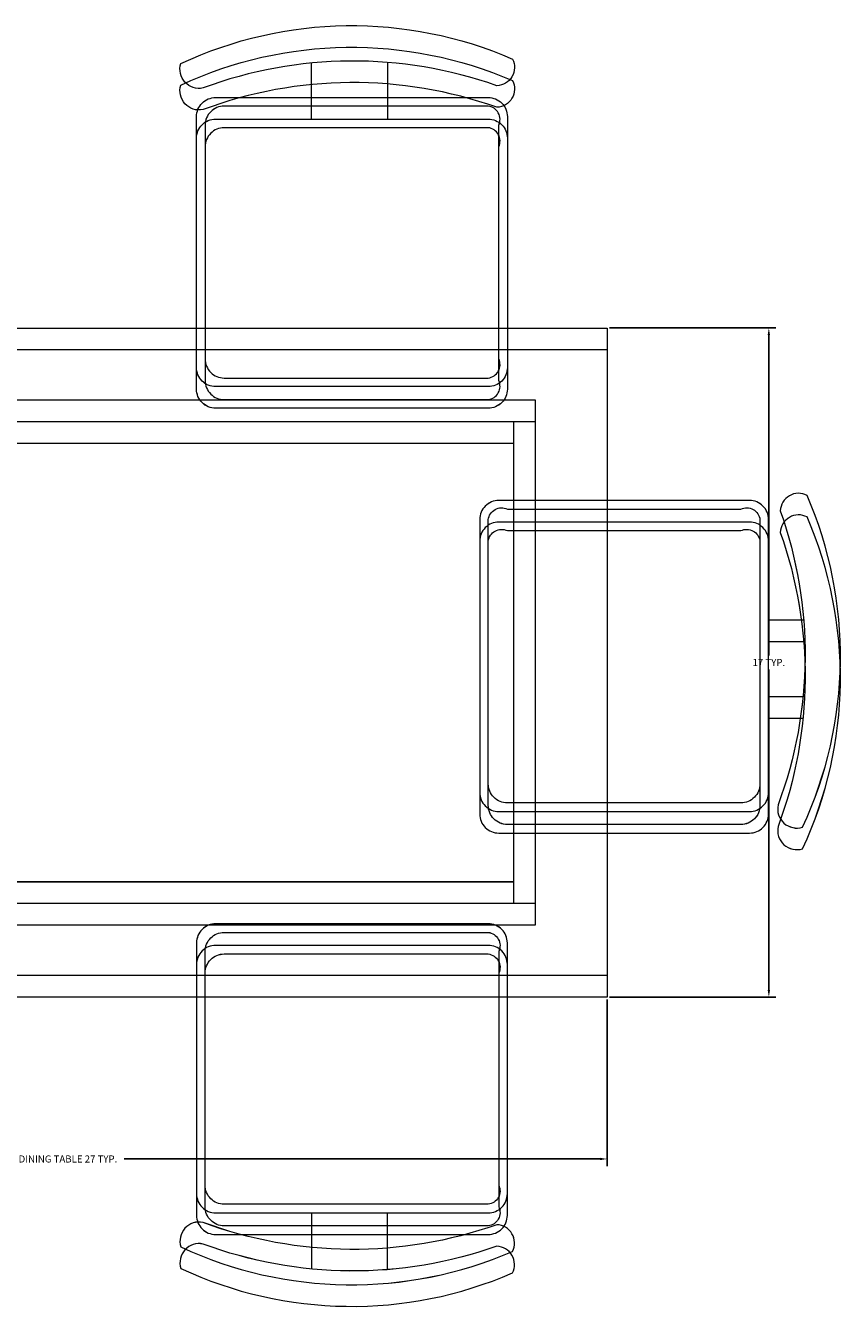
# Model space of a CAD drawing. Units: inches. Extents: x 2168 to 3056, y 1130 to 2629.
# Tile 14 of 42: x 2758 to 2778, y 1971 to 2003. Entities that reach past the tile are written whole.
import ezdxf

# ---------------------------------------------------------------- set-up
doc = ezdxf.new("R2010")
doc.units = ezdxf.units.IN
doc.layers.add('A-ANNO-DIMS', color=2, linetype='Continuous', lineweight=18)
doc.layers.add('A-FURN', color=8, linetype='Continuous', lineweight=13)
doc.styles.get("Standard").update_dxf_attribs({"font": 'arial.ttf'})
doc.dimstyles.get("Standard").update_dxf_attribs({"dimtxt": 0.18, "dimasz": 0.18, "dimexe": 0.18, "dimexo": 0.0625, "dimgap": 0.09, "dimtad": 0, "dimtih": 1, "dimtoh": 1, "dimdec": 4, "dimzin": 0, "dimdsep": 46, "dimtxsty": 'Standard', "dimcen": 0.09, "dimadec": 0, "dimazin": 0, "dimtfac": 1, "dimtdec": 4, "dimtofl": 0, "dimtmove": 0, "dimatfit": 3, "dimfxl": 1, "dimtolj": 1, "dimtzin": 0, "dimarcsym": 0})

# ---------------------------------------------------------------- blocks, each defined once
blk = doc.blocks.new('TABLE-DINING')
for points in [[(0, 17.016), (27.446, 17.016), (27.446, 0.549), (0, 0.549)], [(0, 17.016), (27.446, 17.016), (27.446, 0.549), (0, 0.549)], [(0, 16.467), (27.446, 16.467), (27.446, 0), (0, 0)], [(0, 16.467), (27.446, 16.467), (27.446, 0), (0, 0)], [(1.83, 15.187), (25.616, 15.187), (25.616, 2.379), (1.83, 2.379)], [(1.83, 15.186), (25.616, 15.186), (25.616, 2.378), (1.83, 2.378)], [(1.83, 14.638), (25.616, 14.638), (25.616, 1.83), (1.83, 1.83)], [(1.83, 14.637), (25.616, 14.637), (25.616, 1.829), (1.83, 1.829)], [(2.379, 14.638), (25.067, 14.638), (25.067, 2.928), (2.379, 2.928)], [(2.379, 14.637), (25.067, 14.637), (25.067, 2.927), (2.379, 2.927)], [(2.379, 14.089), (25.067, 14.089), (25.067, 2.379), (2.379, 2.379)], [(2.379, 14.089), (25.067, 14.089), (25.067, 2.378), (2.379, 2.378)]]:
    blk.add_lwpolyline(points, close=True)
blk = doc.blocks.new('*D24')
at = {"layer": 'A-ANNO-DIMS', "color": 0, "lineweight": -2, "transparency": 16777216}
for p, q in [((2744.965, 1978.514), (2744.965, 1974.279)), ((2772.411, 1978.514), (2772.411, 1974.279)), ((2745.145, 1974.459), (2757.257, 1974.459)), ((2772.231, 1974.459), (2760.12, 1974.459))]:
    blk.add_line(p, q, dxfattribs=at)
at = {"layer": 'A-ANNO-DIMS', "color": 0, "transparency": 16777216}
for points in [[(2745.145, 1974.489), (2745.145, 1974.429), (2744.965, 1974.459)], [(2772.231, 1974.489), (2772.231, 1974.429), (2772.411, 1974.459)]]:
    blk.add_solid(points, dxfattribs=at)
at = {"layer": 'Defpoints', "color": 0, "transparency": 16777216}
for p in [(2744.965, 1978.576), (2772.411, 1978.576), (2772.411, 1974.459)]:
    blk.add_point(p, dxfattribs=at)
at = {"layer": 'A-ANNO-DIMS', "color": 0, "transparency": 16777216, "insert": (2758.688, 1974.459), "char_height": 0.18, "attachment_point": 5}
blk.add_mtext('\\A1;DINING TABLE 27 TYP.', dxfattribs=at)
blk = doc.blocks.new('*D25')
at = {"layer": 'A-ANNO-DIMS', "color": 0, "lineweight": -2, "transparency": 16777216}
for p, q in [((2772.474, 1995.593), (2776.708, 1995.593)), ((2776.528, 1995.413), (2776.528, 1987.265)), ((2776.528, 1978.756), (2776.528, 1986.904)), ((2772.474, 1978.576), (2776.708, 1978.576))]:
    blk.add_line(p, q, dxfattribs=at)
at = {"layer": 'A-ANNO-DIMS', "color": 0, "transparency": 16777216}
for points in [[(2776.498, 1995.413), (2776.558, 1995.413), (2776.528, 1995.593)], [(2776.498, 1978.756), (2776.558, 1978.756), (2776.528, 1978.576)]]:
    blk.add_solid(points, dxfattribs=at)
at = {"layer": 'Defpoints', "color": 0, "transparency": 16777216}
for p in [(2772.411, 1995.593), (2776.528, 1995.593), (2772.411, 1978.576)]:
    blk.add_point(p, dxfattribs=at)
at = {"layer": 'A-ANNO-DIMS', "color": 0, "transparency": 16777216, "insert": (2776.528, 1987.085), "char_height": 0.18, "attachment_point": 5}
blk.add_mtext('\\A1;17 TYP.', dxfattribs=at)

msp = doc.modelspace()

# ---------------------------------------------------------------- linework, layer by layer
at = {"layer": 'A-FURN'}
for points in [[(2762.129, 2001.697, -0.578392), (2761.563, 2002.32, -0.214524), (2770.001, 2002.433, -0.552014), (2769.604, 2001.754, 0.175809), (2762.129, 2001.697)], [(2762.129, 2001.697, -0.578392), (2761.563, 2002.32, -0.214524), (2770.001, 2002.433, -0.552014), (2769.604, 2001.754, 0.175809), (2762.129, 2001.697)], [(2762.129, 2001.148, -0.578392), (2761.563, 2001.771, -0.214524), (2770.001, 2001.884, -0.552014), (2769.604, 2001.205, 0.175809), (2762.129, 2001.148)], [(2762.129, 2001.148, -0.578392), (2761.563, 2001.771, -0.214524), (2770.001, 2001.884, -0.552014), (2769.604, 2001.205, 0.175809), (2762.129, 2001.148)], [(2764.884, 2001.454), (2764.884, 2002.332, 0.064759)], [(2764.884, 2001.454), (2764.884, 2002.331, 0.064759)], [(2764.884, 2000.905), (2764.884, 2001.783, 0.064759)], [(2764.884, 2000.905), (2764.884, 2001.782, 0.064759)], [(2769.386, 2001.454, -0.414214), (2769.872, 2000.968), (2769.872, 1994.587, -0.414214), (2769.386, 1994.102), (2762.446, 1994.102, -0.414214), (2761.961, 1994.587), (2761.961, 2000.968, -0.414214), (2762.446, 2001.454), (2769.386, 2001.454)], [(2769.386, 2001.454, -0.414214), (2769.872, 2000.968), (2769.872, 1994.587, -0.414214), (2769.386, 1994.101), (2762.446, 1994.101, -0.414214), (2761.961, 1994.587), (2761.961, 2000.968, -0.414214), (2762.446, 2001.454), (2769.386, 2001.454)], [(2769.386, 2000.905, -0.414214), (2769.872, 2000.419), (2769.872, 1994.038, -0.414214), (2769.386, 1993.553), (2762.446, 1993.553, -0.414214), (2761.961, 1994.038), (2761.961, 2000.419, -0.414214), (2762.446, 2000.905), (2769.386, 2000.905)], [(2769.386, 2000.905, -0.414214), (2769.872, 2000.419), (2769.872, 1994.038, -0.414214), (2769.386, 1993.552), (2762.446, 1993.552, -0.414214), (2761.961, 1994.038), (2761.961, 2000.419, -0.414214), (2762.446, 2000.905), (2769.386, 2000.905)], [(2776.52, 1990.721, 0.414214), (2776.035, 1991.207), (2769.654, 1991.207, 0.414214), (2769.168, 1990.721), (2769.168, 1983.781, 0.414214), (2769.654, 1983.296), (2776.035, 1983.296, 0.414214), (2776.52, 1983.781), (2776.52, 1990.721)], [(2776.52, 1990.721, 0.414214), (2776.035, 1991.206), (2769.654, 1991.206, 0.414214), (2769.168, 1990.721), (2769.168, 1983.781, 0.414214), (2769.654, 1983.295), (2776.035, 1983.295, 0.414214), (2776.52, 1983.781), (2776.52, 1990.721)], [(2776.82, 1990.94, -0.175809), (2776.764, 1983.464, 0.578392), (2777.386, 1982.898, 0.214524), (2777.5, 1991.336, 0.552014), (2776.82, 1990.94, -0.065079)], [(2776.82, 1990.939, -0.175809), (2776.764, 1983.464, 0.578392), (2777.387, 1982.898, 0.214524), (2777.5, 1991.336, 0.552014), (2776.82, 1990.939, -0.065079)], [(2776.82, 1990.391, -0.175809), (2776.764, 1982.915, 0.578392), (2777.386, 1982.349, 0.214524), (2777.5, 1990.787, 0.552014), (2776.82, 1990.391, -0.065079)], [(2776.82, 1990.39, -0.175809), (2776.764, 1982.915, 0.578392), (2777.387, 1982.349, 0.214524), (2777.5, 1990.787, 0.552014), (2776.82, 1990.39, -0.065079)], [(2776.52, 1990.172, 0.414214), (2776.035, 1990.658), (2769.654, 1990.658, 0.414214), (2769.168, 1990.172), (2769.168, 1983.232, 0.414214), (2769.654, 1982.747), (2776.035, 1982.747, 0.414214), (2776.52, 1983.232), (2776.52, 1990.172)], [(2776.52, 1990.172, 0.414214), (2776.035, 1990.658), (2769.654, 1990.658, 0.414214), (2769.168, 1990.172), (2769.168, 1983.232, 0.414214), (2769.654, 1982.747), (2776.035, 1982.747, 0.414214), (2776.52, 1983.232), (2776.52, 1990.172)], [(2776.52, 1986.219), (2777.398, 1986.219, -0.064759)], [(2776.52, 1986.219), (2777.398, 1986.219, -0.064759)], [(2776.52, 1985.67), (2777.398, 1985.67, -0.064759)], [(2776.52, 1985.67), (2777.398, 1985.67, -0.064759)], [(2769.386, 1973.088, 0.414214), (2769.872, 1973.574), (2769.872, 1979.955, 0.414214), (2769.386, 1980.44), (2762.446, 1980.44, 0.414214), (2761.961, 1979.955), (2761.961, 1973.574, 0.414214), (2762.446, 1973.088), (2769.386, 1973.088)], [(2769.386, 1973.088, 0.414214), (2769.872, 1973.573), (2769.872, 1979.954, 0.414214), (2769.386, 1980.44), (2762.446, 1980.44, 0.414214), (2761.961, 1979.954), (2761.961, 1973.573, 0.414214), (2762.446, 1973.088), (2769.386, 1973.088)], [(2769.386, 1972.539, 0.414214), (2769.872, 1973.025), (2769.872, 1979.406, 0.414214), (2769.386, 1979.891), (2762.446, 1979.891, 0.414214), (2761.961, 1979.406), (2761.961, 1973.025, 0.414214), (2762.446, 1972.539), (2769.386, 1972.539)], [(2769.386, 1972.539, 0.414214), (2769.872, 1973.024), (2769.872, 1979.406, 0.414214), (2769.386, 1979.891), (2762.446, 1979.891, 0.414214), (2761.961, 1979.406), (2761.961, 1973.024, 0.414214), (2762.446, 1972.539), (2769.386, 1972.539)], [(2764.884, 1973.088), (2764.884, 1972.21, -0.064759)], [(2764.884, 1973.088), (2764.884, 1972.21, -0.064759)], [(2769.604, 1972.788, -0.175809), (2762.129, 1972.845, 0.578392), (2761.563, 1972.222, 0.214524), (2770.001, 1972.109, 0.552014), (2769.604, 1972.788, -0.065079)], [(2769.604, 1972.788, -0.175809), (2762.129, 1972.844, 0.578392), (2761.563, 1972.222, 0.214524), (2770.001, 1972.108, 0.552014), (2769.604, 1972.788, -0.065079)], [(2769.604, 1972.239, -0.175809), (2762.129, 1972.296, 0.578392), (2761.563, 1971.673, 0.214524), (2770.001, 1971.56, 0.552014), (2769.604, 1972.239, -0.065079)], [(2769.604, 1972.239, -0.175809), (2762.129, 1972.295, 0.578392), (2761.563, 1971.673, 0.214524), (2770.001, 1971.56, 0.552014), (2769.604, 1972.239, -0.065079)], [(2764.884, 1972.539), (2764.884, 1971.661, -0.064759)], [(2764.884, 1972.539), (2764.884, 1971.661, -0.064759)]]:
    msp.add_lwpolyline(points, format="xyb", dxfattribs=at)
for points in [[(2766.826, 2002.347), (2766.826, 2001.454)], [(2766.826, 2002.347), (2766.826, 2001.454)], [(2766.826, 2001.799), (2766.826, 2000.905)], [(2766.826, 2001.798), (2766.826, 2000.905)], [(2777.414, 1988.162), (2776.52, 1988.162)], [(2777.414, 1988.161), (2776.52, 1988.161)], [(2777.414, 1987.613), (2776.52, 1987.613)], [(2777.414, 1987.612), (2776.52, 1987.612)], [(2766.826, 1972.194), (2766.826, 1973.088)], [(2766.826, 1972.194), (2766.826, 1973.088)], [(2766.826, 1971.646), (2766.826, 1972.539)], [(2766.826, 1971.645), (2766.826, 1972.539)]]:
    msp.add_lwpolyline(points, dxfattribs=at)
for points in [[(2769.383, 2001.235), (2762.665, 2001.235, 0.414214), (2762.179, 2000.75), (2762.179, 1994.806, 0.414214), (2762.665, 1994.32), (2769.383, 1994.32, 0.512069), (2769.653, 1994.806), (2769.653, 2000.75, 0.512069)], [(2769.383, 2001.235), (2762.665, 2001.235, 0.414214), (2762.179, 2000.749), (2762.179, 1994.806, 0.414214), (2762.665, 1994.32), (2769.383, 1994.32, 0.512069), (2769.653, 1994.806), (2769.653, 2000.749, 0.512069)], [(2769.383, 2000.686), (2762.665, 2000.686, 0.414214), (2762.179, 2000.201), (2762.179, 1994.257, 0.414214), (2762.665, 1993.771), (2769.383, 1993.771, 0.512069), (2769.653, 1994.257), (2769.653, 2000.201, 0.512069)], [(2769.383, 2000.686), (2762.665, 2000.686, 0.414214), (2762.179, 2000.2), (2762.179, 1994.257, 0.414214), (2762.665, 1993.771), (2769.383, 1993.771, 0.512069), (2769.653, 1994.257), (2769.653, 2000.2, 0.512069)], [(2776.302, 1990.718), (2776.302, 1984, -0.414214), (2775.816, 1983.514), (2769.872, 1983.514, -0.414214), (2769.387, 1984), (2769.387, 1990.718, -0.512069), (2769.872, 1990.988), (2775.816, 1990.988, -0.512069)], [(2776.302, 1990.718), (2776.302, 1984, -0.414214), (2775.816, 1983.514), (2769.872, 1983.514, -0.414214), (2769.387, 1984), (2769.387, 1990.718, -0.512069), (2769.872, 1990.988), (2775.816, 1990.988, -0.512069)], [(2776.302, 1990.169), (2776.302, 1983.451, -0.414214), (2775.816, 1982.966), (2769.872, 1982.966, -0.414214), (2769.387, 1983.451), (2769.387, 1990.169, -0.512069), (2769.872, 1990.439), (2775.816, 1990.439, -0.512069)], [(2776.302, 1990.169), (2776.302, 1983.451, -0.414214), (2775.816, 1982.965), (2769.872, 1982.965, -0.414214), (2769.387, 1983.451), (2769.387, 1990.169, -0.512069), (2769.872, 1990.439), (2775.816, 1990.439, -0.512069)], [(2769.383, 1973.307), (2762.665, 1973.307, -0.414214), (2762.179, 1973.792), (2762.179, 1979.736, -0.414214), (2762.665, 1980.222), (2769.383, 1980.222, -0.512069), (2769.653, 1979.736), (2769.653, 1973.792, -0.512069)], [(2769.383, 1973.307), (2762.665, 1973.307, -0.414214), (2762.179, 1973.792), (2762.179, 1979.736, -0.414214), (2762.665, 1980.221), (2769.383, 1980.221, -0.512069), (2769.653, 1979.736), (2769.653, 1973.792, -0.512069)], [(2769.383, 1972.758), (2762.665, 1972.758, -0.414214), (2762.179, 1973.243), (2762.179, 1979.187, -0.414214), (2762.665, 1979.673), (2769.383, 1979.673, -0.512069), (2769.653, 1979.187), (2769.653, 1973.243, -0.512069)], [(2769.383, 1972.758), (2762.665, 1972.758, -0.414214), (2762.179, 1973.243), (2762.179, 1979.187, -0.414214), (2762.665, 1979.672), (2769.383, 1979.672, -0.512069), (2769.653, 1979.187), (2769.653, 1973.243, -0.512069)]]:
    msp.add_lwpolyline(points, format="xyb", close=True, dxfattribs=at)

# ---------------------------------------------------------------- block references
msp.add_blockref('TABLE-DINING', (2744.965, 1978.576), dxfattribs=at)

# ---------------------------------------------------------------- dimensions: what is measured, and where the dimension line sits
at = {"layer": 'A-ANNO-DIMS'}
dim = msp.add_linear_dim(base=(2776.528, 1995.593), p1=(2772.411, 1978.576), p2=(2772.411, 1995.593), angle=90, text='<> TYP.', dimstyle='Standard', override={"dimdec": 0, "dimlfac": 1, "dimrnd": 0, "dimzin": 0, "dimdsep": 46, "dimlunit": 2}, dxfattribs=at)
dim.commit()
dim.dimension.update_dxf_attribs({"geometry": '*D25', "text_midpoint": (2776.528, 1987.085)})
dim = msp.add_linear_dim(base=(2772.411, 1974.459), p1=(2744.965, 1978.576), p2=(2772.411, 1978.576), text='DINING TABLE <> TYP.', dimstyle='Standard', override={"dimdec": 0, "dimlfac": 1, "dimrnd": 0, "dimzin": 0, "dimdsep": 46, "dimlunit": 2}, dxfattribs=at)
dim.commit()
dim.dimension.update_dxf_attribs({"geometry": '*D24', "text_midpoint": (2758.688, 1974.459)})

doc.saveas('drawing.dxf')
